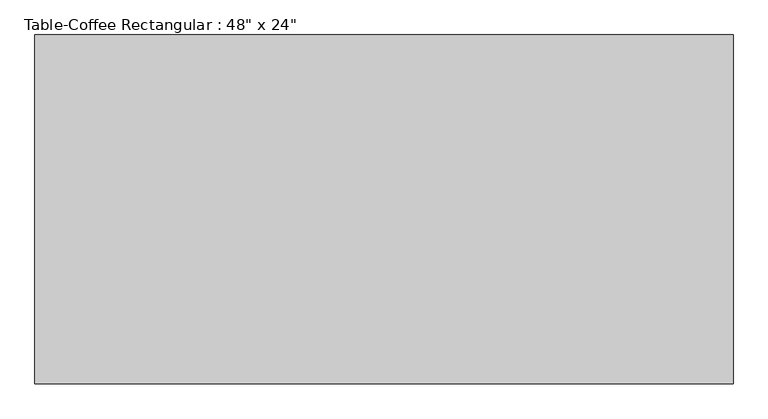
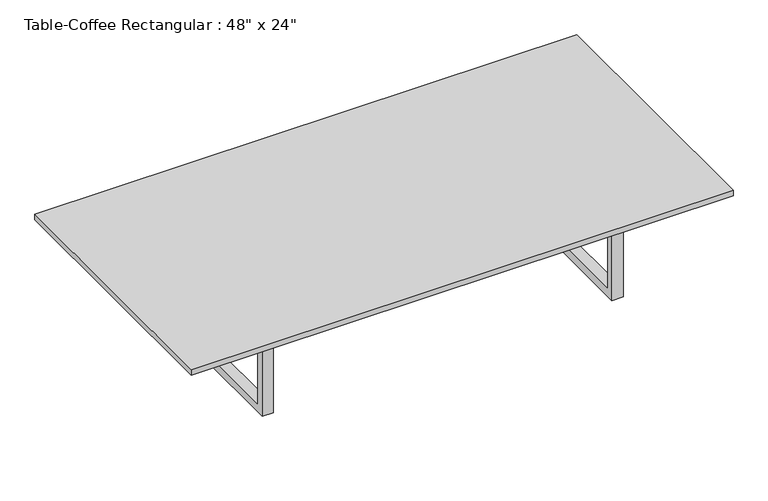
"""IFC4 building model written with IfcOpenShell, lengths in millimetres: furniture geometry."""

from ifc_helpers import new_model, si_unit, frame, origin, place, context, project, spatial, polyline, outline, extrude, source, transform, mapped, element, save


def furniture_0c59c13b(model_context):
    return source(origin(), model_context, "Body", "SweptSolid", [
        extrude(outline(polyline([(1222.9336303, 674.4108318), (1222.9336303, 64.8108318), (3.7336303, 64.8108318), (3.7336303, 674.4108318), (1222.9336303, 674.4108318)])), frame((0.0, 0.0, 215.9), z_axis=(0.0, 0.0, 1.0), x_axis=(1.0, 0.0, 0.0)), (0.0, 0.0, 1.0), 12.7),
        extrude(outline(polyline([(141.0108318, 215.9), (598.2108318, 215.9), (598.2108318, 0.0), (141.0108318, 0.0), (141.0108318, 215.9)]), holes=[polyline([(160.0608318, 196.85), (160.0608318, 19.05), (579.1608318, 19.05), (579.1608318, 196.85), (160.0608318, 196.85)])]), frame((206.9336303, 0.0, 0.0), z_axis=(1.0, 0.0, 0.0), x_axis=(0.0, 1.0, 0.0)), (0.0, 0.0, 1.0), 25.4),
        extrude(outline(polyline([(141.0108318, 215.9), (598.2108318, 215.9), (598.2108318, 0.0), (141.0108318, 0.0), (141.0108318, 215.9)]), holes=[polyline([(160.0608318, 196.85), (160.0608318, 19.05), (579.1608318, 19.05), (579.1608318, 196.85), (160.0608318, 196.85)])]), frame((994.3336303, 0.0, 0.0), z_axis=(1.0, 0.0, 0.0), x_axis=(0.0, 1.0, 0.0)), (0.0, 0.0, 1.0), 25.4),
        extrude(outline(polyline([(994.3336303, 379.1358318), (994.3336303, 360.0858318), (232.3336303, 360.0858318), (232.3336303, 379.1358318), (994.3336303, 379.1358318)])), frame((0.0, 0.0, 196.85), z_axis=(0.0, 0.0, 1.0), x_axis=(1.0, 0.0, 0.0)), (0.0, 0.0, 1.0), 19.05),
    ])


if __name__ == "__main__":
    model = new_model("IFC4")
    model_context = context("Model", 3, world=origin())
    ifc_project = project(units=[si_unit("LENGTHUNIT", "METRE", prefix="MILLI")], contexts=[model_context])
    site = spatial("IfcSite", under=ifc_project)
    building = spatial("IfcBuilding", under=site)
    placement = place(None, origin())
    furniture_shape = furniture_0c59c13b(model_context)
    element("IfcFurniture", 1, ObjectType="Table-Coffee Rectangular : 48\" x 24\"", at=placement, inside=building, context=model_context, shape_type="MappedRepresentation", body=[
        mapped(furniture_shape, transform((0.0, 0.0, 0.0), x_axis=(1.0, 0.0, 0.0), y_axis=(0.0, 1.0, 0.0), z_axis=(0.0, 0.0, 1.0))),
    ])
    save(model, "model.ifc")

# Revit data of these elements
# Type "Table-Coffee Rectangular : 48\" x 24\""
#   Assembly Code = "E2020200"
#   Height = 0' - 9"
#   Length = 4' - 0"
#   Width = 2' - 0"
#   Base Material = Metal - Chrome
#   Table Top Material = Laminate - Ivory,Matte
#   Default Elevation = 0
# Element 1 (IfcFurniture, "Table-Coffee Rectangular : 48\" x 24\"")
#   Materials on its faces: "Metal - Chrome", "Laminate - Ivory,Matte"
# Materials
#   "Metal - Chrome": colour RGB 57 57 57, transparency 0
#   "Laminate - Ivory,Matte": colour RGB 247 247 239, transparency 0
